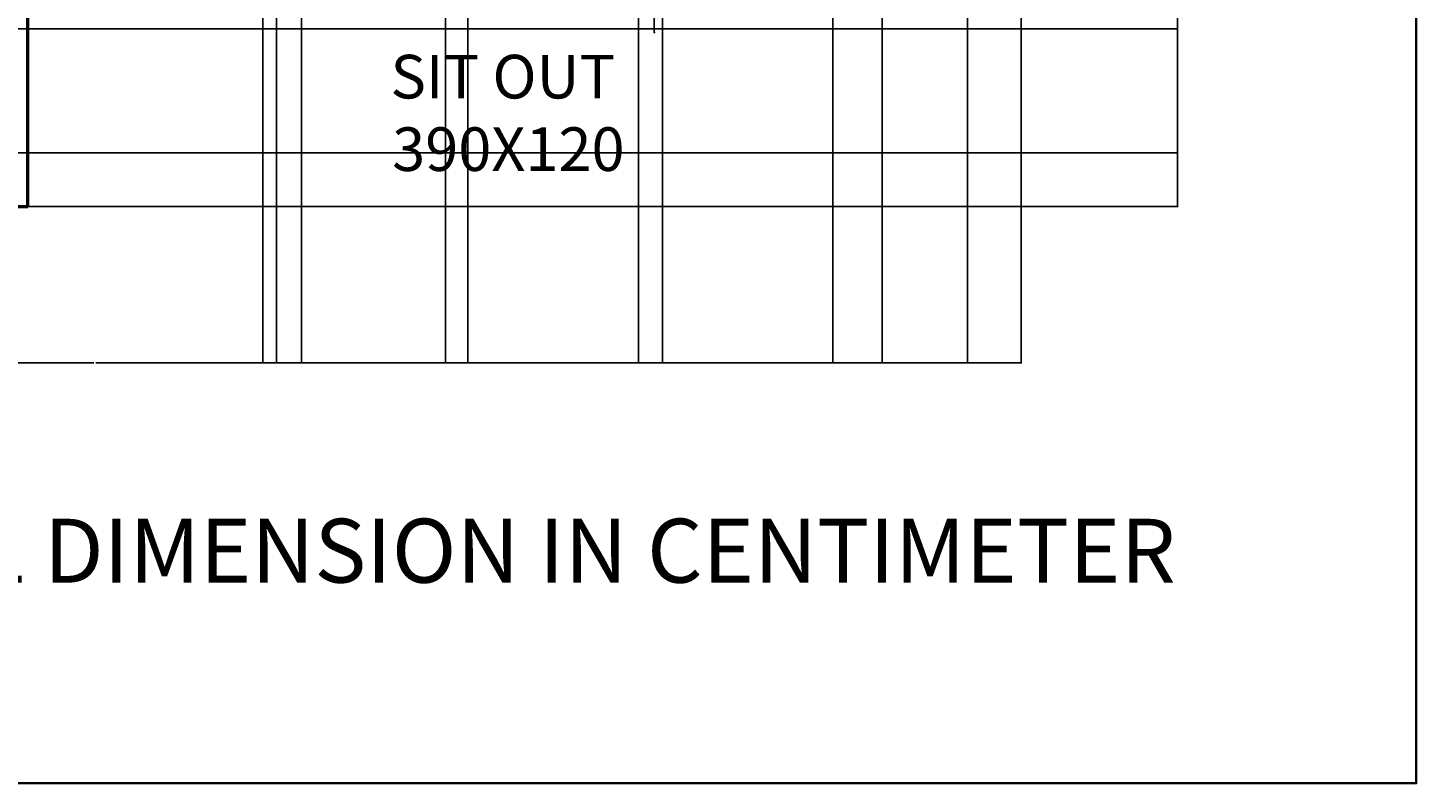
# Model space of a CAD drawing. Units: centimetres. Extents: x 2050 to 3144, y 831 to 2296.
# Tile 2 of 7: x 2553 to 3144, y 831 to 1152. Entities that reach past the tile are written whole.
import ezdxf

# ---------------------------------------------------------------- set-up
doc = ezdxf.new("R2010")
doc.units = ezdxf.units.CM
for name, color, linetype, lineweight in [('A-ANNO-DIMS', 2, 'Continuous', 18), ('A-ANNO-TEXT', 7, 'Continuous', 18), ('A-ANNO-TTLB', 7, 'Continuous', 35), ('A-AREA-IDEN', 7, 'Continuous', 25), ('A-FLOR', 7, 'Continuous', 25), ('A-WALL', 7, 'Continuous', 50)]:
    doc.layers.add(name, color=color, linetype=linetype, lineweight=lineweight)
doc.styles.get("Standard").update_dxf_attribs({"font": 'arial.ttf'})
doc.dimstyles.get("Standard").update_dxf_attribs({"dimtxt": 0.18, "dimasz": 0.18, "dimexe": 0.18, "dimexo": 0.0625, "dimgap": 0.09, "dimtad": 0, "dimtih": 1, "dimtoh": 1, "dimdec": 4, "dimzin": 0, "dimdsep": 46, "dimtxsty": 'Standard', "dimcen": 0.09, "dimadec": 0, "dimazin": 0, "dimtfac": 1, "dimtdec": 4, "dimtofl": 0, "dimtmove": 0, "dimatfit": 3, "dimfxl": 1, "dimtolj": 1, "dimtzin": 0, "dimarcsym": 0})

# ---------------------------------------------------------------- blocks, each defined once
blk = doc.blocks.new('*D31')
at = {"layer": 'A-ANNO-DIMS', "color": 0, "lineweight": -2, "transparency": 16777216}
for p, q in [((2187.01, 1076.25), (2187.01, 1009.53)), ((2975.59, 1076.25), (2975.59, 1009.53)), ((2187.19, 1009.71), (2580.9, 1009.71)), ((2975.41, 1009.71), (2581.69, 1009.71))]:
    blk.add_line(p, q, dxfattribs=at)
at = {"layer": 'A-ANNO-DIMS', "color": 0, "transparency": 16777216}
for points in [[(2187.19, 1009.74), (2187.19, 1009.68), (2187.01, 1009.71)], [(2975.41, 1009.74), (2975.41, 1009.68), (2975.59, 1009.71)]]:
    blk.add_solid(points, dxfattribs=at)
at = {"layer": 'Defpoints', "color": 0, "transparency": 16777216}
for p in [(2187.01, 1076.31), (2975.59, 1076.31), (2975.59, 1009.71)]:
    blk.add_point(p, dxfattribs=at)
at = {"layer": 'A-ANNO-DIMS', "color": 0, "transparency": 16777216, "insert": (2581.3, 1009.71), "char_height": 0.18, "attachment_point": 5}
blk.add_mtext('\\A1;788.6', dxfattribs=at)
blk = doc.blocks.new('*D49')
at = {"layer": 'A-ANNO-DIMS', "color": 0, "lineweight": -2, "transparency": 16777216}
for p, q in [((2669.23, 1188.95), (2669.23, 1009.53)), ((2740.09, 1188.95), (2740.09, 1009.53)), ((2669.41, 1009.71), (2704.27, 1009.71)), ((2739.91, 1009.71), (2705.05, 1009.71))]:
    blk.add_line(p, q, dxfattribs=at)
at = {"layer": 'A-ANNO-DIMS', "color": 0, "transparency": 16777216}
for points in [[(2669.41, 1009.74), (2669.41, 1009.68), (2669.23, 1009.71)], [(2739.91, 1009.74), (2739.91, 1009.68), (2740.09, 1009.71)]]:
    blk.add_solid(points, dxfattribs=at)
at = {"layer": 'Defpoints', "color": 0, "transparency": 16777216}
for p in [(2669.23, 1189.01), (2740.09, 1189.01), (2740.09, 1009.71)]:
    blk.add_point(p, dxfattribs=at)
at = {"layer": 'A-ANNO-DIMS', "color": 0, "transparency": 16777216, "insert": (2704.66, 1009.71), "char_height": 0.18, "attachment_point": 5}
blk.add_mtext('\\A1;70.86', dxfattribs=at)
blk = doc.blocks.new('*D50')
at = {"layer": 'A-ANNO-DIMS', "color": 0, "lineweight": -2, "transparency": 16777216}
for p, q in [((2740.09, 1188.95), (2740.09, 1009.53)), ((2895.36, 1188.95), (2895.36, 1009.53)), ((2740.27, 1009.71), (2817.27, 1009.71)), ((2895.18, 1009.71), (2818.18, 1009.71))]:
    blk.add_line(p, q, dxfattribs=at)
at = {"layer": 'A-ANNO-DIMS', "color": 0, "transparency": 16777216}
for points in [[(2740.27, 1009.74), (2740.27, 1009.68), (2740.09, 1009.71)], [(2895.18, 1009.74), (2895.18, 1009.68), (2895.36, 1009.71)]]:
    blk.add_solid(points, dxfattribs=at)
at = {"layer": 'Defpoints', "color": 0, "transparency": 16777216}
for p in [(2740.09, 1189.01), (2895.36, 1189.01), (2895.36, 1009.71)]:
    blk.add_point(p, dxfattribs=at)
at = {"layer": 'A-ANNO-DIMS', "color": 0, "transparency": 16777216, "insert": (2817.72, 1009.71), "char_height": 0.18, "attachment_point": 5}
blk.add_mtext('\\A1;155.27', dxfattribs=at)
blk = doc.blocks.new('*D57')
at = {"layer": 'A-ANNO-DIMS', "color": 0, "lineweight": -2, "transparency": 16777216}
for p, q in [((2916.44, 1462.1), (2916.44, 1009.53)), ((2952.73, 1440.88), (2952.73, 1009.53)), ((2916.62, 1009.71), (2934.19, 1009.71)), ((2952.55, 1009.71), (2934.98, 1009.71))]:
    blk.add_line(p, q, dxfattribs=at)
at = {"layer": 'A-ANNO-DIMS', "color": 0, "transparency": 16777216}
for points in [[(2916.62, 1009.74), (2916.62, 1009.68), (2916.44, 1009.71)], [(2952.55, 1009.74), (2952.55, 1009.68), (2952.73, 1009.71)]]:
    blk.add_solid(points, dxfattribs=at)
at = {"layer": 'Defpoints', "color": 0, "transparency": 16777216}
for p in [(2916.44, 1462.16), (2952.73, 1440.94), (2952.73, 1009.71)]:
    blk.add_point(p, dxfattribs=at)
at = {"layer": 'A-ANNO-DIMS', "color": 0, "transparency": 16777216, "insert": (2934.58, 1009.71), "char_height": 0.18, "attachment_point": 5}
blk.add_mtext('\\A1;36.29', dxfattribs=at)
blk = doc.blocks.new('*D64')
at = {"layer": 'A-ANNO-DIMS', "color": 0, "lineweight": -2, "transparency": 16777216}
for p, q in [((2975.65, 1189.01), (3042.37, 1189.01)), ((3042.19, 1188.83), (3042.19, 1132.85)), ((3042.19, 1076.49), (3042.19, 1132.48)), ((2975.65, 1076.31), (3042.37, 1076.31))]:
    blk.add_line(p, q, dxfattribs=at)
at = {"layer": 'A-ANNO-DIMS', "color": 0, "transparency": 16777216}
for points in [[(3042.16, 1188.83), (3042.22, 1188.83), (3042.19, 1189.01)], [(3042.16, 1076.49), (3042.22, 1076.49), (3042.19, 1076.31)]]:
    blk.add_solid(points, dxfattribs=at)
at = {"layer": 'Defpoints', "color": 0, "transparency": 16777216}
for p in [(2975.59, 1189.01), (3042.19, 1189.01), (2975.59, 1076.31)]:
    blk.add_point(p, dxfattribs=at)
at = {"layer": 'A-ANNO-DIMS', "color": 0, "transparency": 16777216, "insert": (3042.19, 1132.66), "char_height": 0.18, "attachment_point": 5}
blk.add_mtext('\\A1;112.7', dxfattribs=at)
blk = doc.blocks.new('*D65')
at = {"layer": 'A-ANNO-DIMS', "color": 0, "lineweight": -2, "transparency": 16777216}
for p, q in [((2812.73, 1924.83), (2812.73, 1009.53)), ((2822.89, 1914.67), (2822.89, 1009.53)), ((2812.91, 1009.71), (2817.42, 1009.71)), ((2822.71, 1009.71), (2818.19, 1009.71))]:
    blk.add_line(p, q, dxfattribs=at)
at = {"layer": 'A-ANNO-DIMS', "color": 0, "transparency": 16777216}
for points in [[(2812.91, 1009.74), (2812.91, 1009.68), (2812.73, 1009.71)], [(2822.71, 1009.74), (2822.71, 1009.68), (2822.89, 1009.71)]]:
    blk.add_solid(points, dxfattribs=at)
at = {"layer": 'Defpoints', "color": 0, "transparency": 16777216}
for p in [(2812.73, 1924.89), (2822.89, 1914.73), (2822.89, 1009.71)]:
    blk.add_point(p, dxfattribs=at)
at = {"layer": 'A-ANNO-DIMS', "color": 0, "transparency": 16777216, "insert": (2817.81, 1009.71), "char_height": 0.18, "attachment_point": 5}
blk.add_mtext('\\A1;10.16', dxfattribs=at)
blk = doc.blocks.new('*D67')
at = {"layer": 'A-ANNO-DIMS', "color": 0, "lineweight": -2, "transparency": 16777216}
for p, q in [((2227.86, 1151.97), (3042.37, 1151.97)), ((3042.19, 1151.79), (3042.19, 1125.75)), ((3042.19, 1099.35), (3042.19, 1125.39)), ((2209.93, 1099.17), (3042.37, 1099.17))]:
    blk.add_line(p, q, dxfattribs=at)
at = {"layer": 'A-ANNO-DIMS', "color": 0, "transparency": 16777216}
for points in [[(3042.16, 1151.79), (3042.22, 1151.79), (3042.19, 1151.97)], [(3042.16, 1099.35), (3042.22, 1099.35), (3042.19, 1099.17)]]:
    blk.add_solid(points, dxfattribs=at)
at = {"layer": 'Defpoints', "color": 0, "transparency": 16777216}
for p in [(2227.8, 1151.97), (2209.87, 1099.17), (3042.19, 1099.17)]:
    blk.add_point(p, dxfattribs=at)
at = {"layer": 'A-ANNO-DIMS', "color": 0, "transparency": 16777216, "insert": (3042.19, 1125.57), "char_height": 0.18, "attachment_point": 5}
blk.add_mtext('\\A1;52.79', dxfattribs=at)
blk = doc.blocks.new('*D68')
at = {"layer": 'A-ANNO-DIMS', "color": 0, "lineweight": -2, "transparency": 16777216}
for p, q in [((2652.73, 1914.67), (2652.73, 1009.53)), ((2730.58, 1841.3), (2730.58, 1009.53)), ((2652.91, 1009.71), (2691.26, 1009.71)), ((2730.4, 1009.71), (2692.05, 1009.71))]:
    blk.add_line(p, q, dxfattribs=at)
at = {"layer": 'A-ANNO-DIMS', "color": 0, "transparency": 16777216}
for points in [[(2652.91, 1009.74), (2652.91, 1009.68), (2652.73, 1009.71)], [(2730.4, 1009.74), (2730.4, 1009.68), (2730.58, 1009.71)]]:
    blk.add_solid(points, dxfattribs=at)
at = {"layer": 'Defpoints', "color": 0, "transparency": 16777216}
for p in [(2652.73, 1914.73), (2730.58, 1841.36), (2730.58, 1009.71)]:
    blk.add_point(p, dxfattribs=at)
at = {"layer": 'A-ANNO-DIMS', "color": 0, "transparency": 16777216, "insert": (2691.65, 1009.71), "char_height": 0.18, "attachment_point": 5}
blk.add_mtext('\\A1;77.85', dxfattribs=at)
blk = doc.blocks.new('*D73')
at = {"layer": 'A-ANNO-DIMS', "color": 0, "lineweight": -2, "transparency": 16777216}
for p, q in [((2658.57, 1971.45), (2658.57, 1009.53)), ((2652.73, 1924.83), (2652.73, 1009.53)), ((2652.91, 1009.71), (2655.26, 1009.71)), ((2658.39, 1009.71), (2656.04, 1009.71))]:
    blk.add_line(p, q, dxfattribs=at)
at = {"layer": 'A-ANNO-DIMS', "color": 0, "transparency": 16777216}
for points in [[(2652.91, 1009.74), (2652.91, 1009.68), (2652.73, 1009.71)], [(2658.39, 1009.74), (2658.39, 1009.68), (2658.57, 1009.71)]]:
    blk.add_solid(points, dxfattribs=at)
at = {"layer": 'Defpoints', "color": 0, "transparency": 16777216}
for p in [(2658.57, 1971.51), (2652.73, 1924.89), (2658.57, 1009.71)]:
    blk.add_point(p, dxfattribs=at)
at = {"layer": 'A-ANNO-DIMS', "color": 0, "transparency": 16777216, "insert": (2655.65, 1009.71), "char_height": 0.18, "attachment_point": 5}
blk.add_mtext('\\A1;5.847', dxfattribs=at)
blk = doc.blocks.new('*D74')
at = {"layer": 'A-ANNO-DIMS', "color": 0, "lineweight": -2, "transparency": 16777216}
for p, q in [((2952.73, 2064.83), (2952.73, 1009.53)), ((2822.89, 2004.16), (2822.89, 1009.53)), ((2823.07, 1009.71), (2887.35, 1009.71)), ((2952.55, 1009.71), (2888.26, 1009.71))]:
    blk.add_line(p, q, dxfattribs=at)
at = {"layer": 'A-ANNO-DIMS', "color": 0, "transparency": 16777216}
for points in [[(2823.07, 1009.74), (2823.07, 1009.68), (2822.89, 1009.71)], [(2952.55, 1009.74), (2952.55, 1009.68), (2952.73, 1009.71)]]:
    blk.add_solid(points, dxfattribs=at)
at = {"layer": 'Defpoints', "color": 0, "transparency": 16777216}
for p in [(2952.73, 2064.89), (2822.89, 2004.22), (2952.73, 1009.71)]:
    blk.add_point(p, dxfattribs=at)
at = {"layer": 'A-ANNO-DIMS', "color": 0, "transparency": 16777216, "insert": (2887.81, 1009.71), "char_height": 0.18, "attachment_point": 5}
blk.add_mtext('\\A1;129.84', dxfattribs=at)
blk = doc.blocks.new('*D77')
at = {"layer": 'A-ANNO-DIMS', "color": 0, "lineweight": -2, "transparency": 16777216}
for p, q in [((2819.23, 1348.09), (2819.41, 1348.09)), ((2819.32, 1348), (2819.32, 1348.18)), ((2819.32, 1150.35), (2819.32, 1224.32)), ((2819.5, 1150.35), (2819.32, 1150.35))]:
    blk.add_line(p, q, dxfattribs=at)
at = {"layer": 'A-ANNO-DIMS', "color": 0, "transparency": 16777216}
blk.add_solid([(2819.35, 1224.32), (2819.29, 1224.32), (2819.32, 1224.5)], dxfattribs=at)
at = {"layer": 'Defpoints', "color": 0, "transparency": 16777216}
for p in [(2819.32, 1348.09), (2819.32, 1224.5)]:
    blk.add_point(p, dxfattribs=at)
at = {"layer": 'A-ANNO-DIMS', "color": 0, "transparency": 16777216, "insert": (2820.05, 1150.35), "char_height": 0.18, "attachment_point": 5}
blk.add_mtext('\\A1;R123.59', dxfattribs=at)

msp = doc.modelspace()

# ---------------------------------------------------------------- linework, layer by layer
at = {"layer": 'A-ANNO-TTLB'}
msp.add_lwpolyline([(2050.3641, 2295.8578), (3143.7558, 2295.8578), (3143.7558, 830.6902), (2050.3641, 830.6902)], close=True, dxfattribs=at)
at = {"layer": 'A-FLOR'}
for p in [(2975.5865, 1551.8748), (2552.7265, 1076.3148)]:
    msp.add_line(p, (2975.5865, 1076.3148), dxfattribs=at)
at = {"layer": 'A-WALL'}
for p, q in [((2552.7265, 1076.3148), (2552.7265, 1442.0348)), ((2187.0065, 1076.3148), (2552.7265, 1076.3148))]:
    msp.add_line(p, q, dxfattribs=at)

# ---------------------------------------------------------------- texts
at = {"layer": 'A-ANNO-TEXT'}
msp.add_text('ALL DIMENSION IN CENTIMETER', height=27.192544, dxfattribs=at).set_placement((2488.3592, 916.1363))
at = {"layer": 'A-AREA-IDEN'}
for s, p in [('SIT OUT', (2707.1226, 1122.3437)), ('390X120', (2707.8394, 1091.463))]:
    msp.add_text(s, height=18.57938, dxfattribs=at).set_placement(p)

# ---------------------------------------------------------------- dimensions: what is measured, and where the dimension line sits
at = {"layer": 'A-ANNO-DIMS'}
for base, p1, p2, override, picture, middle in [((2952.7265, 1009.7148), (2822.8865, 2004.2202), (2952.7265, 2064.8948), {"dimdec": 2, "dimlfac": 1, "dimrnd": 0, "dimzin": 0, "dimdsep": 46, "dimlunit": 2}, '*D74', (2887.8065, 1009.7148)), ((2658.5737, 1009.7148), (2652.7265, 1924.8948), (2658.5737, 1971.5118), {"dimdec": 3, "dimlfac": 1, "dimrnd": 0, "dimzin": 0, "dimdsep": 46, "dimlunit": 2}, '*D73', (2655.6501, 1009.7148)), ((2822.8865, 1009.7148), (2812.7265, 1924.8948), (2822.8865, 1914.7348), {"dimdec": 2, "dimlfac": 1, "dimrnd": 0, "dimzin": 0, "dimdsep": 46, "dimlunit": 2}, '*D65', (2817.8065, 1009.7148)), ((2730.579, 1009.7148), (2652.7265, 1914.7348), (2730.579, 1841.3577), {"dimdec": 2, "dimlfac": 1, "dimrnd": 0, "dimzin": 0, "dimdsep": 46, "dimlunit": 2}, '*D68', (2691.6528, 1009.7148)), ((2952.7265, 1009.7148), (2916.4375, 1462.1606), (2952.7265, 1440.9424), {"dimdec": 2, "dimlfac": 1, "dimrnd": 0, "dimzin": 0, "dimdsep": 46, "dimlunit": 2}, '*D57', (2934.582, 1009.7148)), ((2740.0885, 1009.7148), (2669.2319, 1189.0148), (2740.0885, 1189.0148), {"dimdec": 2, "dimlfac": 1, "dimrnd": 0, "dimzin": 0, "dimdsep": 46, "dimlunit": 2}, '*D49', (2704.6602, 1009.7148)), ((2895.3598, 1009.7148), (2740.0885, 1189.0148), (2895.3598, 1189.0148), {"dimdec": 2, "dimlfac": 1, "dimrnd": 0, "dimzin": 0, "dimdsep": 46, "dimlunit": 2}, '*D50', (2817.7241, 1009.7148)), ((2975.5865, 1009.7148), (2187.0065, 1076.3148), (2975.5865, 1076.3148), {"dimdec": 1, "dimlfac": 1, "dimrnd": 0, "dimzin": 0, "dimdsep": 46, "dimlunit": 2}, '*D31', (2581.2965, 1009.7148))]:
    dim = msp.add_linear_dim(base=base, p1=p1, p2=p2, dimstyle='Standard', override=override, dxfattribs=at)
    dim.commit()
    dim.dimension.update_dxf_attribs({"geometry": picture, "text_midpoint": middle})
dim = msp.add_radius_dim(center=(2819.3175, 1348.0853), mpoint=(2819.318, 1224.4996), dimstyle='Standard', override={"dimdec": 2, "dimlfac": 1, "dimrnd": 0, "dimzin": 0, "dimdsep": 46, "dimlunit": 2}, dxfattribs=at)
dim.commit()
dim.dimension.update_dxf_attribs({"geometry": '*D77', "text_midpoint": (2820.0482, 1150.3483), "dimtype": 164})
for base, p1, p2, override, picture, middle in [((3042.1865, 1189.0148), (2975.5865, 1076.3148), (2975.5865, 1189.0148), {"dimdec": 1, "dimlfac": 1, "dimrnd": 0, "dimzin": 0, "dimdsep": 46, "dimlunit": 2}, '*D64', (3042.1865, 1132.6648)), ((3042.1865, 1099.1748), (2227.7996, 1151.9671), (2209.8665, 1099.1748), {"dimdec": 2, "dimlfac": 1, "dimrnd": 0, "dimzin": 0, "dimdsep": 46, "dimlunit": 2}, '*D67', (3042.1865, 1125.5709))]:
    dim = msp.add_linear_dim(base=base, p1=p1, p2=p2, angle=90, dimstyle='Standard', override=override, dxfattribs=at)
    dim.commit()
    dim.dimension.update_dxf_attribs({"geometry": picture, "text_midpoint": middle})

doc.saveas('drawing.dxf')
